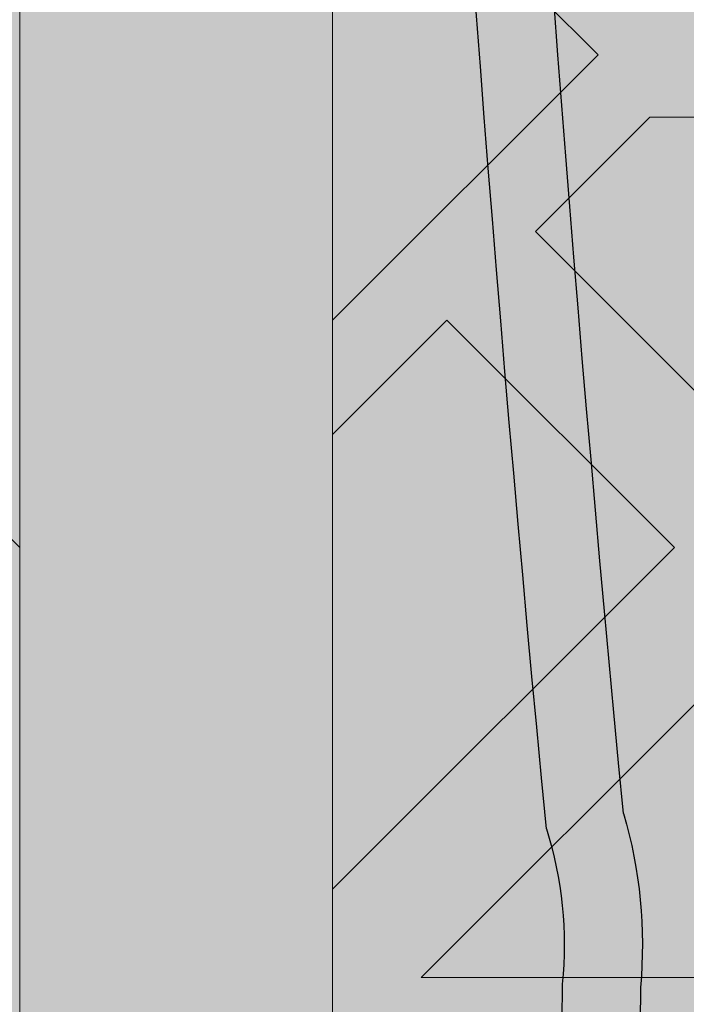
# Model space of a CAD drawing. Units: inches. Extents: x 844 to 2234, y 346 to 1084.
# Tile 70 of 93: x 1998.757 to 2000.116, y 694.327 to 696.335. Entities that reach past the tile are written whole.
import ezdxf

# ---------------------------------------------------------------- set-up
doc = ezdxf.new("R2010")
doc.units = ezdxf.units.IN
doc.header["$MEASUREMENT"] = 0
for name, color, linetype, lineweight in [('A-ANNO-DIMS', 2, 'Continuous', 18), ('furniture', 8, 'Continuous', 18), ('RA-AP-01$0$INT', 35, 'Continuous', 5)]:
    doc.layers.add(name, color=color, linetype=linetype, lineweight=lineweight)
doc.layers.add('RA-AP-01$0$FURN', color=3, linetype='Continuous')
doc.layers.add('RA-AP-01$0$WOOD', color=64, linetype='Continuous')
doc.styles.get("Standard").update_dxf_attribs({"font": 'arial.ttf'})
doc.dimstyles.get("Standard").update_dxf_attribs({"dimtxt": 6, "dimasz": 3, "dimexe": 0.18, "dimexo": 0.0625, "dimgap": 0.09, "dimtad": 0, "dimtih": 1, "dimtoh": 1, "dimdec": 1, "dimzin": 0, "dimdsep": 46, "dimlunit": 3, "dimtxsty": 'Standard', "dimblk": 'ARCHTICK', "dimcen": 0.09, "dimadec": 0, "dimazin": 0, "dimtfac": 1, "dimtdec": 1, "dimtofl": 0, "dimtmove": 0, "dimatfit": 3, "dimfxl": 1, "dimtolj": 1, "dimtzin": 0, "dimarcsym": 0})

# ---------------------------------------------------------------- blocks, each defined once
blk = doc.blocks.new('A$C18D01794')
at = {"layer": 'RA-AP-01$0$INT'}
h = blk.add_hatch(color=256, dxfattribs=at)
h.paths.add_polyline_path([(4.469348592586677, -7.07085414521094), (4.505206456958073, -7.03499628085108), (4.505206456958071, -7.106712009593861)])
h.paths.add_polyline_path([(4.455206456960671, -7.084996280832395), (4.476922185709333, -7.106712009588038), (4.433490728198045, -7.106712009588038)])
h.paths.add_polyline_path([(4.405206456958073, -7.034996280813718), (4.441064321339218, -7.070854145206393), (4.40520645695807, -7.106712009576003)])
h.paths.add_polyline_path([(4.425206456989053, -6.911460746921742), (4.455206456990736, -6.881460746929706), (4.485206456989055, -6.911460746937677), (4.48520645696979, -7.026712009590022), (4.455206456965227, -7.056712009584936), (4.425206456969784, -7.026712009579853)])
h.paths.add_polyline_path([(4.505206456958073, -6.831460746955388), (4.505206456958071, -6.903176475661116), (4.469348592616738, -6.867318611308251)])
h.paths.add_polyline_path([(4.425206456964688, -6.707925213036777), (4.455206456964794, -6.677925213027025), (4.485206456964689, -6.707925213017265), (4.485206456983951, -6.823176475683938), (4.455206456990736, -6.853176475686799), (4.425206456983956, -6.823176475689667)])
h.paths.add_polyline_path([(4.425206456974126, -6.504389679118949), (4.455206456959092, -6.474389679124341), (4.485206456974132, -6.504389679129721), (4.485206456993396, -6.619640941768059), (4.45520645699153, -6.649640941779566), (4.425206456993394, -6.619640941791077)])
h.paths.add_polyline_path([(4.46934859260189, -6.663783077416661), (4.505206456958071, -6.627925213048953), (4.505206456958073, -6.699640941761311)])
h.paths.add_polyline_path([(4.405206456958073, -6.627925213005104), (4.441064321354427, -6.663783077389926), (4.405206456958072, -6.699640941797813)])
h.paths.add_polyline_path([(4.405206456958072, -6.424389679139403), (4.441064321333084, -6.460247543502882), (4.405206456958072, -6.496105407889427)])
h.paths.add_polyline_path([(4.469348592580547, -6.460247543498336), (4.505206456958071, -6.424389679109282), (4.505206456958071, -6.496105407864332)])
h.paths.add_polyline_path([(4.425206456957888, -6.300854145208262), (4.45520645695415, -6.270854145221655), (4.485206456959507, -6.300854145217359), (4.48520645695824, -6.416105407863534), (4.455206456954537, -6.44610540787688), (4.425206456957888, -6.416105407889874)])
h.paths.add_polyline_path([(4.425206456957888, -6.226712009591025), (4.471064321332215, -6.226712009591025), (4.425206456957888, -6.272569873980103)])
h.paths.add_polyline_path([(4.499348592575121, -6.226712009591029), (4.636064321343707, -6.226712009591025), (4.666064321342317, -6.256712009589254), (4.636064321340932, -6.286712009591028), (4.499348592588945, -6.286712009591028), (4.469348592591685, -6.256712009584116)])
h.paths.add_polyline_path([(4.680206456964641, -6.270854145214393), (4.716064321337824, -6.306712009588038), (4.644348592591454, -6.306712009588038)])
h.paths.add_polyline_path([(4.644348592588108, -6.206712009588038), (4.716064321341167, -6.206712009588038), (4.680206456964637, -6.242569873964111)])
h.paths.add_polyline_path([(4.724348592586768, -6.226712009589824), (4.861064321340514, -6.226712009589824), (4.891064321340324, -6.256712009589255), (4.861064321340141, -6.286712009589827), (4.724348592587134, -6.286712009589821), (4.694348592586957, -6.256712009589254)])
h.paths.add_polyline_path([(4.905206456964143, -6.270854145212892), (4.941064321338827, -6.306712009588038), (4.869348592589457, -6.306712009588039)])
h.paths.add_polyline_path([(4.869348592586113, -6.206712009588038), (4.941064321342172, -6.206712009588038), (4.905206456964145, -6.242569873965612)])
h.paths.add_polyline_path([(4.949348592587774, -6.226712009589824), (5.086064321341521, -6.226712009589824), (5.116064321341329, -6.256712009589252), (5.08606432134115, -6.286712009589823), (4.949348592588145, -6.286712009589827), (4.919348592587961, -6.256712009589255)])
h.paths.add_polyline_path([(5.130206456963645, -6.270854145214393), (5.166064321336834, -6.306712009588038), (5.094348592590464, -6.306712009588038)])
h.paths.add_polyline_path([(5.094348592587119, -6.206712009588038), (5.166064321340178, -6.206712009588038), (5.130206456963651, -6.242569873964107)])
h.paths.add_polyline_path([(5.174348592584578, -6.226712009591027), (5.311064321353163, -6.226712009591027), (5.341064321336602, -6.256712009584116), (5.31106432133934, -6.286712009591028), (5.174348592587352, -6.286712009591028), (5.144348592585969, -6.256712009589254)])
h.paths.add_polyline_path([(5.325206456968778, -6.300854145217359), (5.355206456974136, -6.270854145221653), (5.385206456970396, -6.300854145208262), (5.385206456970396, -6.416105407889878), (5.355206456973747, -6.44610540787688), (5.325206456970044, -6.416105407863533)])
h.paths.add_polyline_path([(5.339348592596073, -6.226712009591029), (5.385206456970396, -6.226712009591025), (5.385206456970398, -6.272569873980105)])
h.paths.add_polyline_path([(5.325206456954155, -6.504389679129722), (5.355206456969194, -6.474389679124342), (5.38520645695416, -6.504389679118949), (5.385206456934896, -6.619640941791077), (5.355206456936758, -6.649640941779564), (5.325206456934888, -6.619640941768057)])
h.paths.add_polyline_path([(5.305206456958072, -6.424389679097139), (5.341064321347739, -6.460247543498338), (5.305206456958072, -6.496105407876472)])
h.paths.add_polyline_path([(5.369348592595204, -6.460247543502882), (5.40520645695807, -6.42438967915155), (5.405206456958072, -6.496105407877278)])
h.paths.add_polyline_path([(5.405206456958072, -6.627925213017245), (5.405206456958072, -6.69964094178567), (5.369348592573857, -6.663783077389926)])
h.paths.add_polyline_path([(5.305206456958072, -6.62792521303681), (5.341064321326393, -6.663783077416663), (5.305206456958072, -6.69964094177345)])
h.paths.add_polyline_path([(5.325206456963599, -6.707925213017267), (5.355206456963494, -6.677925213027021), (5.385206456963598, -6.707925213036775), (5.385206456944334, -6.823176475689665), (5.355206456937552, -6.853176475686797), (5.325206456944333, -6.823176475683936)])
h.paths.add_polyline_path([(5.305206456958072, -6.831460746943246), (5.341064321311551, -6.867318611308252), (5.305206456958072, -6.903176475673257)])
h.paths.add_polyline_path([(5.325206456939231, -6.911460746937672), (5.355206456937552, -6.881460746929707), (5.385206456939235, -6.911460746921742), (5.385206456958502, -7.026712009579853), (5.355206456963061, -7.056712009584934), (5.3252064569585, -7.026712009590026)])
h.paths.add_polyline_path([(5.404581768715993, -6.832085435167151, 0.001217816984214), (5.405206456958072, -6.832312009593747), (5.405206456958072, -6.90317647569123), (5.369348592563558, -6.867318611308251)])
h.paths.add_polyline_path([(5.36934859258907, -7.070854145206393), (5.40520645695807, -7.034996280825861), (5.405206456958072, -7.106712009563858)])
h.paths.add_polyline_path([(5.355206456967613, -7.084996280832394), (5.376922185730239, -7.106712009588038), (5.333490728218953, -7.106712009588036)])
h.paths.add_polyline_path([(5.30520645695807, -7.034996280838937), (5.341064321341609, -7.070854145210942), (5.305206456958074, -7.106712009606006)])
h = blk.add_hatch(color=256, dxfattribs=at)
h.paths.add_polyline_path([(4.505206456958071, -6.627925213048953), (4.46934859260189, -6.663783077416663), (4.505206456958071, -6.699640941761309), (4.505206456958071, -6.831460746955389), (4.469348592616735, -6.867318611308252), (4.505206456958071, -6.903176475661112), (4.505206456958071, -7.03499628085108), (4.469348592586679, -7.070854145210939), (4.505206456952245, -7.106712009588038), (4.476922185709333, -7.106712009588038), (4.455206456960671, -7.084996280832395), (4.433490728198047, -7.106712009588038), (4.405206456946033, -7.10671200958804), (4.441064321339216, -7.070854145206393), (4.40520645695807, -7.034996280813718), (4.405206456958072, -6.903176475703379), (4.441064321364728, -6.867318611308251), (4.40520645695807, -6.83146074691313), (4.40520645695807, -6.699640941797813), (4.441064321354429, -6.663783077389924), (4.405206456958072, -6.627925213005102), (4.405206456958072, -6.496105407889425), (4.441064321333084, -6.460247543502882), (4.405206456958072, -6.424389679139403), (4.405206456958072, -6.206712009588038), (4.644348592588106, -6.206712009588038), (4.680206456964639, -6.242569873964107), (4.716064321341165, -6.206712009588038), (4.869348592586113, -6.206712009588038), (4.905206456964143, -6.24256987396561), (4.941064321342174, -6.206712009588038), (5.094348592587118, -6.206712009588038), (5.130206456963649, -6.242569873964107), (5.166064321340178, -6.206712009588038), (5.405206456958072, -6.206712009588038), (5.405206456958072, -6.42438967915155), (5.369348592595202, -6.46024754350288), (5.40520645695807, -6.49610540787728), (5.40520645695807, -6.627925213017247), (5.369348592573859, -6.663783077389926), (5.40520645695807, -6.699640941785666), (5.40520645695807, -6.831460746925273), (5.36934859256356, -6.867318611308252), (5.405206456958072, -6.90317647569123), (5.405206456958072, -7.034996280825859), (5.369348592589068, -7.070854145206395), (5.405206456982249, -7.106712009588038), (5.376922185730244, -7.106712009588038), (5.355206456967613, -7.084996280832397), (5.333490728218955, -7.106712009588036), (5.305206456976043, -7.106712009588035), (5.341064321341609, -7.07085414521094), (5.305206456958072, -7.034996280838935), (5.305206456958072, -6.90317647567326), (5.34106432131155, -6.867318611308252), (5.305206456958072, -6.831460746943244), (5.30520645695807, -6.699640941773452), (5.341064321326395, -6.663783077416663), (5.305206456958072, -6.627925213036814), (5.305206456958072, -6.496105407876472), (5.341064321347738, -6.46024754349834), (5.305206456958072, -6.424389679097137), (5.30520645695807, -6.306712009588038), (5.166064321336834, -6.306712009588038), (5.130206456963647, -6.270854145214393), (5.094348592590464, -6.306712009588038), (4.941064321338827, -6.306712009588036), (4.905206456964145, -6.270854145212892), (4.869348592589459, -6.306712009588038), (4.716064321337822, -6.306712009588036), (4.680206456964641, -6.270854145214393), (4.644348592591453, -6.306712009588038), (4.505206456958071, -6.306712009588038), (4.505206456958071, -6.424389679109282), (4.469348592580545, -6.460247543498338), (4.505206456958071, -6.496105407864328)])
h.paths.add_polyline_path([(4.485206456974132, -6.504389679129722), (4.45520645695909, -6.474389679124341), (4.425206456974128, -6.504389679118945), (4.425206456993394, -6.619640941791079), (4.45520645699153, -6.649640941779566), (4.485206456993396, -6.619640941768059)], flags=16)
h.paths.add_polyline_path([(4.455206456954537, -6.44610540787688), (4.485206456958242, -6.416105407863534), (4.48520645695951, -6.30085414521736), (4.45520645695415, -6.270854145221653), (4.425206456957888, -6.300854145208264), (4.425206456957888, -6.41610540788988)], flags=16)
h.paths.add_polyline_path([(4.455206456964794, -6.677925213027025), (4.42520645696469, -6.707925213036777), (4.425206456983954, -6.82317647568967), (4.455206456990734, -6.853176475686797), (4.485206456983953, -6.823176475683936), (4.485206456964687, -6.707925213017265)], flags=16)
h.paths.add_polyline_path([(4.499348592588947, -6.286712009591028), (4.636064321340932, -6.286712009591028), (4.666064321342317, -6.256712009589254), (4.636064321343707, -6.226712009591027), (4.499348592575121, -6.226712009591029), (4.469348592591685, -6.256712009584118)], flags=16)
h.paths.add_polyline_path([(4.425206456957888, -6.272569873980103), (4.471064321332215, -6.226712009591025), (4.425206456957888, -6.226712009591025)], flags=16)
h.paths.add_polyline_path([(4.455206456990734, -6.881460746929709), (4.425206456989053, -6.91146074692174), (4.425206456969784, -7.026712009579853), (4.455206456965226, -7.056712009584932), (4.485206456969787, -7.026712009590026), (4.485206456989053, -6.911460746937672)], flags=16)
h.paths.add_polyline_path([(4.72434859258714, -6.286712009589821), (4.861064321340141, -6.286712009589829), (4.891064321340324, -6.256712009589254), (4.861064321340513, -6.226712009589823), (4.724348592586768, -6.226712009589823), (4.694348592586956, -6.256712009589254)], flags=16)
h.paths.add_polyline_path([(4.919348592587961, -6.256712009589254), (4.949348592588145, -6.286712009589827), (5.08606432134115, -6.286712009589823), (5.116064321341327, -6.256712009589254), (5.086064321341519, -6.226712009589824), (4.949348592587774, -6.226712009589824)], flags=16)
h.paths.add_polyline_path([(5.144348592585967, -6.256712009589254), (5.174348592587358, -6.286712009591028), (5.311064321339338, -6.286712009591028), (5.3410643213366, -6.256712009584118), (5.311064321353163, -6.226712009591029), (5.174348592584576, -6.226712009591027)], flags=16)
h.paths.add_polyline_path([(5.32520645693489, -6.619640941768055), (5.355206456936755, -6.649640941779566), (5.385206456934894, -6.619640941791079), (5.38520645695416, -6.504389679118949), (5.355206456969194, -6.474389679124341), (5.325206456954153, -6.504389679129724)], flags=16)
h.paths.add_polyline_path([(5.325206456970042, -6.416105407863534), (5.355206456973747, -6.44610540787688), (5.385206456970398, -6.416105407889876), (5.385206456970398, -6.30085414520826), (5.355206456974136, -6.270854145221653), (5.325206456968778, -6.30085414521736)], flags=16)
h.paths.add_polyline_path([(5.325206456963599, -6.707925213017265), (5.325206456944333, -6.823176475683936), (5.355206456937552, -6.853176475686797), (5.385206456944332, -6.823176475689667), (5.385206456963596, -6.707925213036773), (5.355206456963492, -6.677925213027027)], flags=16)
h.paths.add_polyline_path([(5.32520645693923, -6.911460746937674), (5.3252064569585, -7.026712009590026), (5.355206456963062, -7.056712009584934), (5.3852064569585, -7.026712009579853), (5.385206456939234, -6.911460746921738), (5.355206456937552, -6.881460746929707)], flags=16)
h.paths.add_polyline_path([(5.339348592596071, -6.226712009591029), (5.385206456970398, -6.272569873980103), (5.385206456970396, -6.226712009591027)], flags=16)
blk.add_hatch(color=256, dxfattribs=at).paths.add_polyline_path([(4.505206456958071, -6.306712009588038), (5.305206456958072, -6.306712009588038), (5.305206456958072, -7.106712009588038), (5.255206456951893, -7.10671200958804), (5.25520645694868, -6.356712009605972), (4.555206456959269, -6.356712009587461), (4.555206456956052, -7.106712009588038), (4.505206456958073, -7.106712009588038)])
h = blk.add_hatch(color=256, dxfattribs=at)
h.paths.add_polyline_path([(4.585917135068448, -6.356712009588273), (4.614201406330596, -6.356712009589021), (4.668846067270487, -6.411356670531338), (4.723490728212344, -6.356712009591912), (4.771774999457151, -6.35671200959319), (4.826419660396886, -6.411356670535356), (4.862780050090322, -6.374996280843536), (4.844495778842715, -6.356712009595112), (4.862780050090411, -6.356712009595595), (4.905206456960182, -6.399138416468211), (4.947632863832445, -6.356712009597838), (4.965917135079675, -6.356712009598322), (4.947632863831759, -6.374996280845421), (4.983993253523576, -6.411356670538857), (5.038637914464627, -6.356712009600247), (5.08692218571208, -6.356712009601523), (5.141566846649976, -6.411356670541852), (5.196211507589851, -6.356712009604411), (5.224495778822615, -6.356712009605161), (4.905206456953975, -6.676001331473793)])
h.paths.add_polyline_path([(4.895206456956031, -6.637717060225675), (4.895206456958921, -6.528427738347902), (4.840561796018589, -6.583072399285802)], flags=16)
h.paths.add_polyline_path([(4.915206456955638, -6.637717060226121), (4.969851117895509, -6.583072399288678), (4.915206456957609, -6.528427738348344)], flags=16)
h.paths.add_polyline_path([(4.826419660395175, -6.568930263661755), (4.881064321335613, -6.514285602723745), (4.771774999456703, -6.514285602720857)], flags=16)
h.paths.add_polyline_path([(4.983993253519558, -6.568930263665262), (5.038637914460456, -6.514285602726792), (4.929348592581548, -6.514285602724816)], flags=16)
h.paths.add_polyline_path([(4.881064321336025, -6.494285602723742), (4.826419660397532, -6.439640941782821), (4.771774999457062, -6.494285602720859)], flags=16)
h.paths.add_polyline_path([(4.929348592582019, -6.494285602724817), (5.038637914460982, -6.494285602726792), (4.983993253522945, -6.439640941786327)], flags=16)
h.paths.add_polyline_path([(4.895206456960191, -6.480143467100443), (4.895206456962115, -6.407422687715913), (4.876922185715016, -6.389138416467584), (4.840561796021581, -6.425498806159401)], flags=16)
h.paths.add_polyline_path([(4.915206456958487, -6.480143467100889), (4.969851117899527, -6.425498806162279), (4.933490728206909, -6.389138416468043), (4.9152064569598, -6.40742268771434)], flags=16)
h.paths.add_polyline_path([(4.757632863832376, -6.480143467096812), (4.812277524772842, -6.425498806158772), (4.757632863834348, -6.370854145217844)], flags=16)
h.paths.add_polyline_path([(4.737632863832376, -6.480143467096286), (4.737632863834348, -6.370854145217375), (4.682988202893906, -6.425498806155385)], flags=16)
h.paths.add_polyline_path([(5.05278005008503, -6.480143467103376), (5.052780050087917, -6.370854145224413), (4.998135389146995, -6.425498806162908)], flags=16)
h.paths.add_polyline_path([(5.072780050085024, -6.480143467103744), (5.127424711025931, -6.42549880616527), (5.072780050087916, -6.370854145224832)], flags=16)
h.paths.add_polyline_path([(4.935917135072783, -6.706712009592292), (5.255206456948811, -6.387422687716309), (5.255206456948932, -6.415706958964177), (5.200561796010279, -6.470351619902839), (5.255206456949403, -6.524996280841948), (5.25520645694961, -6.5732805520894), (5.200561796009787, -6.627925213029239), (5.236922185702417, -6.664285602721864), (5.255206456949919, -6.646001331474357), (5.255206456949998, -6.664285602721898), (5.212780050078687, -6.706712009592262), (5.25520645695036, -6.749138416463932), (5.255206456950438, -6.767422687711313), (5.236922185702424, -6.749138416463297), (5.200561796009796, -6.785498806155928), (5.255206456950753, -6.840143467096874), (5.25520645695096, -6.888427738341682), (5.200561796010322, -6.943072399282328), (5.255206456951428, -6.997717060223427), (5.255206456951547, -7.026001331471006)])
h.paths.add_polyline_path([(5.042988202883395, -6.785498806155427), (5.097632863823085, -6.840143467095101), (5.097632863822622, -6.730854145216193)], flags=16)
h.paths.add_polyline_path([(5.028846067259663, -6.771356670531693), (5.083490728198774, -6.716712009592573), (4.974201406321001, -6.716712009593042)], flags=16)
h.paths.add_polyline_path([(5.117632863823087, -6.840143467095186), (5.172277524762331, -6.785498806155926), (5.11763286382262, -6.730854145216225)], flags=16)
h.paths.add_polyline_path([(5.08349072819877, -6.696712009593886), (5.028846067259652, -6.642067348654775), (4.974201406320998, -6.696712009593438)], flags=16)
h.paths.add_polyline_path([(5.131774999446817, -6.854285602718917), (5.186419660386065, -6.799640941779662), (5.241064321325782, -6.854285602719365)], flags=17)
h.paths.add_polyline_path([(5.131774999446228, -6.716712009592374), (5.186419660386065, -6.771356670532194), (5.222780050079488, -6.734996280838764), (5.204495778832781, -6.716712009592063)], flags=16)
h.paths.add_polyline_path([(5.097632863822613, -6.682569873970264), (5.097632863823061, -6.573280552091354), (5.042988202883383, -6.627925213031044)], flags=16)
h.paths.add_polyline_path([(5.131774999446899, -6.874285602718915), (5.241064321325809, -6.874285602719364), (5.186419660386591, -6.928930263658598)], flags=17)
h.paths.add_polyline_path([(5.131774999446226, -6.696712009594078), (5.204495778830767, -6.696712009594374), (5.22278005007868, -6.67842773834687), (5.186419660386049, -6.642067348654249)], flags=16)
h.paths.add_polyline_path([(5.11763286382262, -6.682569873970225), (5.17227752476232, -6.627925213030515), (5.117632863823064, -6.573280552091267)], flags=16)
h.paths.add_polyline_path([(5.186419660386069, -6.613783077405491), (5.241064321325754, -6.559138416465795), (5.131774999446791, -6.559138416466263)], flags=16)
h.paths.add_polyline_path([(5.131774999446872, -6.539138416466263), (5.24106432132578, -6.539138416465794), (5.186419660386554, -6.484493755526573)], flags=16)
h.paths.add_polyline_path([(5.255206456951811, -7.08742268770861), (5.255206456951895, -7.106712009588038), (4.555206456956052, -7.106712009588038), (4.555206456956136, -7.087422687708617), (4.905206456953973, -6.737422687710788)])
h.paths.add_polyline_path([(4.983993253513404, -6.8444937555241), (4.92934859257295, -6.899138416462108), (5.03863791445186, -6.899138416465014)], flags=16)
h.paths.add_polyline_path([(4.969851117889988, -6.83035161990006), (4.915206456952556, -6.775706958960171), (4.915206456949648, -6.884996280837944)], flags=16)
h.paths.add_polyline_path([(4.929348592572535, -6.919138416462105), (4.983993253511019, -6.973783077403037), (5.038637914451496, -6.919138416465012)], flags=16)
h.paths.add_polyline_path([(5.052780050074912, -6.93328055208906), (4.998135389134438, -6.987925213027088), (5.052780050072919, -7.042569873968025)], flags=16)
h.paths.add_polyline_path([(5.07278005007491, -6.933280552089588), (5.072780050072918, -7.042569873968497), (5.127424711013374, -6.987925213030498)], flags=16)
h.paths.add_polyline_path([(4.89520645695295, -6.775706958959721), (4.840561796013067, -6.830351619897157), (4.895206456950961, -6.884996280837494)], flags=16)
h.paths.add_polyline_path([(4.915206456948365, -6.933280552085403), (4.915206456946434, -7.006001331471951), (4.933490728192729, -7.024285602719066), (4.969851117886972, -6.987925213026453)], flags=16)
h.paths.add_polyline_path([(4.881064321327021, -6.899138416461022), (4.82641966038902, -6.84449375552057), (4.771774999448108, -6.899138416459029)], flags=16)
h.paths.add_polyline_path([(4.895206456950073, -6.933280552084951), (4.840561796009022, -6.987925213023558), (4.876922185700835, -7.024285602716997), (4.895206456948749, -7.006001331469487)], flags=16)
h.paths.add_polyline_path([(4.983993253510392, -7.0020673486505), (4.947632863816944, -7.038427738342319), (4.965917135064043, -7.05671200959023), (5.038637914448995, -7.056712009591555)], flags=16)
h.paths.add_polyline_path([(4.881064321326543, -6.91913841646102), (4.771774999447578, -6.919138416459031), (4.826419660385607, -6.973783077399508)], flags=16)
h.paths.add_polyline_path([(4.905206456946447, -7.014285602717636), (4.862780050074785, -7.056712009588352), (4.947632863816685, -7.056712009589775)], flags=16)
h.paths.add_polyline_path([(5.14156684663679, -7.002067348654549), (5.086922185696452, -7.056712009592438), (5.196211507574223, -7.056712009594425)], flags=16)
h.paths.add_polyline_path([(4.8264196603837, -7.002067348646972), (4.771774999442643, -7.056712009585575), (4.8444957788276, -7.056712009587508), (4.862780050075511, -7.038427738340416)], flags=16)
h.paths.add_polyline_path([(4.812277524760289, -6.98792521302292), (4.757632863822258, -6.933280552082447), (4.757632863819352, -7.042569873961408)], flags=16)
h.paths.add_polyline_path([(4.73763286382226, -6.933280552082079), (4.682988202881349, -6.987925213020536), (4.737632863819352, -7.04256987396099)], flags=16)
h.paths.add_polyline_path([(4.723490728195188, -7.056712009584289), (4.668846067257299, -7.002067348643949), (4.614201406317417, -7.056712009581383)], flags=16)
h.paths.add_polyline_path([(4.597632863829262, -6.706712009592262), (4.555206456957951, -6.664285602721896), (4.555206456958029, -6.646001331474357), (4.573490728205535, -6.664285602721864), (4.609851117898167, -6.627925213029238), (4.555206456958338, -6.573280552089402), (4.555206456958546, -6.524996280841952), (4.60985111789767, -6.470351619902839), (4.555206456959015, -6.415706958964177), (4.555206456959138, -6.387422687716309), (4.874495778835167, -6.70671200959229), (4.5552064569564, -7.026001331471015), (4.555206456956523, -6.997717060223433), (4.609851117897629, -6.94307239928233), (4.555206456956988, -6.888427738341681), (4.555206456957198, -6.840143467096881), (4.609851117898153, -6.78549880615593), (4.573490728205528, -6.749138416463297), (4.555206456957507, -6.76742268771132), (4.555206456957585, -6.749138416463933)])
h.paths.add_polyline_path([(4.712780050085332, -6.730854145216195), (4.712780050084863, -6.840143467095105), (4.767424711024555, -6.785498806155427)], flags=16)
h.paths.add_polyline_path([(4.726922185709173, -6.716712009592573), (4.781566846648288, -6.771356670531693), (4.836211507586949, -6.716712009593043)], flags=16)
h.paths.add_polyline_path([(4.692780050085327, -6.730854145216225), (4.638135389145619, -6.785498806155928), (4.692780050084865, -6.840143467095185)], flags=16)
h.paths.add_polyline_path([(4.726922185709182, -6.696712009593886), (4.836211507586949, -6.696712009593436), (4.7815668466483, -6.642067348654773)], flags=16)
h.paths.add_polyline_path([(4.678637914461726, -6.71671200959237), (4.605917135075169, -6.716712009592063), (4.587632863828464, -6.734996280838766), (4.623993253521887, -6.771356670532195)], flags=16)
h.paths.add_polyline_path([(4.712780050085336, -6.68256987397026), (4.767424711024568, -6.627925213031042), (4.71278005008489, -6.573280552091352)], flags=16)
h.paths.add_polyline_path([(4.678637914461726, -6.696712009594076), (4.623993253521899, -6.642067348654247), (4.587632863829271, -6.67842773834687), (4.605917135077185, -6.696712009594376)], flags=16)
h.paths.add_polyline_path([(4.692780050085336, -6.682569873970228), (4.692780050084889, -6.573280552091267), (4.638135389145632, -6.627925213030515)], flags=16)
h.paths.add_polyline_path([(4.623993253521885, -6.799640941779662), (4.678637914461131, -6.854285602718915), (4.56934859258217, -6.854285602719365)], flags=17)
h.paths.add_polyline_path([(4.623993253521901, -6.613783077405509), (4.678637914461158, -6.559138416466263), (4.569348592582195, -6.559138416465795)], flags=16)
h.paths.add_polyline_path([(4.678637914461051, -6.874285602718915), (4.623993253521361, -6.928930263658598), (4.569348592582143, -6.874285602719364)], flags=17)
h.paths.add_polyline_path([(4.678637914461076, -6.539138416466263), (4.623993253521399, -6.484493755526573), (4.569348592582167, -6.539138416465796)], flags=16)
h = blk.add_hatch(color=256, dxfattribs=at)
h.paths.add_polyline_path([(5.028846067259997, -6.642067348655121), (4.974201406321342, -6.696712009593783), (5.083490728199115, -6.69671200959423)])
h.paths.add_polyline_path([(4.974201406321344, -6.716712009593388), (5.028846067260004, -6.771356670532039), (5.083490728199117, -6.716712009592919)])
h.paths.add_polyline_path([(5.042988202883738, -6.785498806155768), (5.097632863823428, -6.840143467095449), (5.097632863822963, -6.73085414521654)])
h.paths.add_polyline_path([(5.117632863822961, -6.730854145216568), (5.117632863823428, -6.840143467095531), (5.172277524762674, -6.785498806156272)])
h.paths.add_polyline_path([(5.131774999446572, -6.716712009592718), (5.186419660386406, -6.77135667053254), (5.222780050079831, -6.734996280839116), (5.204495778833122, -6.716712009592409)])
h.paths.add_polyline_path([(5.236922185702764, -6.749138416463644), (5.200561796010139, -6.785498806156274), (5.255206456949971, -6.840143467096101), (5.255206456950271, -6.76742268771115)])
h.paths.add_polyline_path([(5.186419660386412, -6.799640941780006), (5.131774999447164, -6.854285602719262), (5.241064321326123, -6.854285602719711)])
h.paths.add_polyline_path([(5.131774999447238, -6.874285602719261), (5.186419660386934, -6.928930263658944), (5.241064321326153, -6.874285602719709)])
h.paths.add_polyline_path([(5.200561796010663, -6.943072399282675), (5.255206456949324, -6.997717060221329), (5.255206456949777, -6.888427738343558)])
h.paths.add_polyline_path([(5.21278005007903, -6.706712009592607), (5.255206456950223, -6.749138416463798), (5.255206456950696, -6.664285602721891)])
h.paths.add_polyline_path([(5.13177499944657, -6.696712009594424), (5.204495778831106, -6.696712009594723), (5.222780050079024, -6.678427738347219), (5.186419660386397, -6.642067348654592)])
h.paths.add_polyline_path([(5.117632863823405, -6.573280552091611), (5.117632863822955, -6.682569873970578), (5.172277524762665, -6.627925213030859)])
h.paths.add_polyline_path([(5.042988202883727, -6.627925213031387), (5.097632863822957, -6.682569873970603), (5.097632863823407, -6.573280552091697)])
h.paths.add_polyline_path([(5.131774999447135, -6.559138416466609), (5.186419660386394, -6.613783077405857), (5.241064321326097, -6.559138416466144)])
h.paths.add_polyline_path([(5.200561796010128, -6.627925213029584), (5.236922185702758, -6.664285602722211), (5.255206456950264, -6.646001331474705), (5.255206456949948, -6.573280552089752)])
h.paths.add_polyline_path([(5.186419660386895, -6.484493755526919), (5.131774999447213, -6.539138416466609), (5.241064321326127, -6.539138416466142)])
h.paths.add_polyline_path([(5.200561796010624, -6.470351619903183), (5.255206456949745, -6.524996280842298), (5.255206456949276, -6.415706958964523)])
for p, q in [((5.255206456951895, -7.106712009588038), (5.255206456948681, -6.356712009605972)), ((5.131774999446792, -6.559138416466263), (5.241064321325755, -6.559138416465795)), ((5.241064321325755, -6.559138416465795), (5.186419660386049, -6.613783077405509)), ((5.255206456949605, -6.573280552089405), (5.200561796009783, -6.627925213029239)), ((5.255206456949918, -6.646001331474357), (5.255206456949605, -6.573280552089405)), ((5.200561796009783, -6.627925213029238), (5.236922185702415, -6.664285602721863)), ((5.305206456939818, -6.627925213018556), (5.341064321310754, -6.663783077401021)), ((5.186419660386051, -6.642067348654247), (5.222780050078681, -6.67842773834687)), ((5.255206456949919, -6.646001331474357), (5.236922185702415, -6.664285602721864)), ((5.212780050078687, -6.706712009592262), (5.255206456950353, -6.664285602721543)), ((5.25520645694988, -6.74913841646345), (5.255206456950353, -6.664285602721543)), ((5.204495778833082, -6.69671200959206), (5.222780050078681, -6.67842773834687)), ((5.204495778831179, -6.696712009594376), (5.131774999446228, -6.696712009594078)), ((5.212780050078687, -6.706712009592262), (5.25520645694988, -6.74913841646345))]:
    blk.add_line(p, q, dxfattribs=at)
blk.add_lwpolyline([(5.305206456958072, -7.106712009588038), (5.305206456958072, -6.306712009588038), (4.505206456958071, -6.306712009588038), (4.505206456958071, -7.106712009588038)], dxfattribs=at)
blk = doc.blocks.new('A$C32926AE1')
at = {"layer": 'RA-AP-01$0$WOOD'}
h = blk.add_hatch(color=256, dxfattribs=at)
h.dxf.hatch_style = 1
h.paths.add_polyline_path([(5.157430609644524, 4.573483066760929, -0.1009492694046607), (5.155401577623758, 4.593365984175333, -0.1842662638101597), (5.172249623284174, 4.638795604568598, 0.2056608120311276), (5.179560981299304, 4.661316324430096, 0.3614336704623542), (5.134352340494423, 4.706524965234944, 0.2056608120311297), (5.111831620632933, 4.699213607219793, -0.1842662638101113), (5.066402000239693, 4.682365561559342, -0.1055311479399994), (5.045656153913092, 4.68467289944697, 0.1567636581983829), (4.763886414745334, 4.684672899446966, -0.1055311479399895), (4.743140568418733, 4.68236556155934, -0.1842662638100833), (4.6977109480255, 4.69921360721979, 0.2056608120302612), (4.675190228164109, 4.706524965234949, 0.3614336704708441), (4.629981587358889, 4.66131632442871, 0.2056608120245944), (4.637292945374126, 4.638795604567974, -0.1842662638101024), (4.654140991034615, 4.59336598417475, -0.1009492694055169), (4.652111959013835, 4.573483066760181, 0.021410119221476), (4.629748025606143, 4.156712009541676, 0.0214101192214795), (4.652111959013809, 3.739940952323101, -0.1009492694059586), (4.654140991034615, 3.720058034908448, -0.1842662638100975), (4.637292945374126, 3.674628414515226, 0.2056608120245705), (4.629981587358889, 3.652107694654492, 0.3614336704708879), (4.675190228164113, 3.606899053848249, 0.2056608120302384), (4.697710948025501, 3.614210411863408, -0.1842662638100995), (4.743140568418738, 3.63105845752386, -0.1055311479402541), (4.763886414745388, 3.628751119636215, 0.1567636581983776), (5.045656153913137, 3.628751119636244, -0.1055311479397538), (5.066402000239692, 3.631058457523857, -0.1842662638101067), (5.111831620632931, 3.614210411863407, 0.2056608120310924), (5.134352340494417, 3.606899053848256, 0.3614336704624001), (5.179560981299307, 3.652107694653103, 0.2056608120311314), (5.172249623284175, 3.6746284145146, -0.1842662638101402), (5.155401577623758, 3.72005803490786, -0.1009492694051366), (5.15743060964455, 3.739940952322354, 0.0214101192215073), (5.179794543052287, 4.156712009541468, 0.0214101192215252)])
h.paths.add_polyline_path([(4.639748609479751, 4.156712009541513, 0.0213537860821624), (4.661970494867118, 3.741887061152232, -0.094075836301374), (4.664143710413708, 3.7196126951003, -0.1824818158568985), (4.644813765429836, 3.668037719127816, 0.2056608120245319), (4.639939526753007, 3.653023905887301, 0.3614336704710246), (4.676106439397173, 3.616856993242342, 0.2056608120302234), (4.691120252638095, 3.621731231919122, -0.1824818158602558), (4.742695228611606, 3.641061176902986, -0.1029891339458722), (4.766991894714349, 3.638256818950944, 0.156709409989566), (5.042550673941472, 3.638256818950105, -0.102989133958497), (5.066847340047078, 3.641061176902949, -0.1824818158594995), (5.118422316020358, 3.621731231919103, 0.2056608120311416), (5.133436129261316, 3.616856993242346, 0.3614336704621468), (5.169603041905217, 3.653023905886178, 0.2056608120310986), (5.164728803228477, 3.668037719127177, -0.1824818158565612), (5.145398858244737, 3.719612695099578, -0.0940758363009313), (5.147572073791232, 3.741887061151398, 0.0213537860822023), (5.169793959178681, 4.156712009541451, 0.0213537860822226), (5.147572073791203, 4.571536957931898, -0.0940758363005034), (5.145398858244737, 4.59381132398362, -0.1824818158565587), (5.164728803228476, 4.645386299956021, 0.2056608120311045), (5.169603041905216, 4.66040011319702, 0.3614336704621845), (5.133436129261313, 4.696567025840856, 0.2056608120310773), (5.118422316020359, 4.691692787164098, -0.182481815859508), (5.066847340047078, 4.67236284218025, -0.1029891339584606), (5.04255067394148, 4.675167200133092, 0.156709409989566), (4.766991894714357, 4.675167200132257, -0.1029891339458842), (4.742695228611611, 4.672362842180213, -0.1824818158602725), (4.691120252638095, 4.691692787164077, 0.2056608120302152), (4.676106439397174, 4.696567025840858, 0.3614336704710363), (4.639939526753005, 4.660400113195899, 0.2056608120245495), (4.644813765429837, 4.645386299955384, -0.1824818158568934), (4.664143710413708, 4.593811323982902, -0.0940758363009187), (4.661970494867149, 4.571536957931074, 0.021353786082177)], flags=16)
h.paths.add_polyline_path([(5.129794543052235, 4.432167055276933, -0.0141661062790638), (5.130152669293814, 4.156927903047693, -0.0141661062790647), (5.129794543052234, 3.881688750818433, -0.0785247771143638), (5.10979738006795, 3.755143611847103, 0.0945969212073497), (5.105408519571111, 3.717898134952927, 0.1043170707844957), (5.116074640131521, 3.670385395016088, 0.1043170707864965), (5.068561900193738, 3.681051515576561, 0.09459692119553), (5.031316423304057, 3.676662655080835, -0.1580239521427272), (4.778226145355827, 3.676662655080367, 0.0945969211986668), (4.740980668464973, 3.681051515576592, 0.1043170707882822), (4.693467928526415, 3.670385395015844, 0.1043170707867916), (4.704134049087309, 3.717898134953662, 0.0945969211972894), (4.69974518859162, 3.755143611844042, -0.0785247771163196), (4.679748025606343, 3.881688750818406, -0.0141661062790663), (4.679389899364763, 4.156927903047693, -0.0141661062790672), (4.679748025606343, 4.432167055276998, -0.0785247771163064), (4.699745188591625, 4.55871219425134, 0.094596921197333), (4.704134049087308, 4.595957671141738, 0.1043170707867205), (4.693467928526416, 4.643470411079523, 0.1043170707882628), (4.740980668464965, 4.632804290518776, 0.0945969211988114), (4.778226145355874, 4.637193151015016, -0.158023952142669), (5.031316423304015, 4.637193151014546, 0.0945969211956361), (5.068561900193736, 4.632804290518806, 0.1043170707864979), (5.11607464013152, 4.643470411079278, 0.1043170707844617), (5.105408519571112, 4.595957671142455, 0.0945969212074597), (5.109797380067959, 4.558712194248236, -0.0785247771143467)], flags=0)
h.paths.add_polyline_path([(5.119794532311105, 4.432259799204851, -0.0142000800617244), (5.120156169157484, 4.156927903047701, -0.0142000800617277), (5.119794532311105, 3.881596006890482, -0.0784894509520253), (5.100273383573699, 3.758192358677797, 0.0940138827242913), (5.095413455884425, 3.717477693979438, 0.0606271852308753), (5.099615656341024, 3.686844378806616, 0.0606271852322524), (5.068982341167493, 3.691046579263239, 0.0940138827010453), (5.028267676478798, 3.686186651576848, -0.1580706864508061), (4.781274892180912, 3.686186651576435, 0.0940138827026903), (4.740560227491556, 3.691046579263279, 0.0606271852339895), (4.709926912317155, 3.686844378806508, 0.0606271852329405), (4.714129112773991, 3.717477693980356, 0.094013882701304), (4.709269185087677, 3.758192358669163, -0.0784894509577193), (4.689748036347473, 3.881596006890469, -0.014200080061729), (4.689386399501094, 4.156927903047709, -0.0142000800617217), (4.689748036347473, 4.432259799204808, -0.078489450957724), (4.709269185087651, 4.555663447426125, 0.0940138827014585), (4.714129112773992, 4.596378112114996, 0.0606271852329731), (4.709926912317154, 4.62701142728886, 0.0606271852340196), (4.74056022749157, 4.622809226832087, 0.0940138827024997), (4.781274892180847, 4.627669154518912, -0.1580706864508359), (5.028267676478777, 4.627669154518526, 0.0940138827010946), (5.068982341167492, 4.622809226832129, 0.060627185232254), (5.099615656341024, 4.627011427288751, 0.0606271852308727), (5.095413455884425, 4.59637811211593, 0.0940138827241088), (5.100273383573675, 4.555663447417647, -0.0784894509520978)], flags=0)
h.paths.add_polyline_path([(5.06978912287499, 4.430218106756144, -0.014241683694547), (5.070173729147532, 4.156927903047672, -0.0142416836945458), (5.06978912287499, 3.883637699339223, -0.0800609523125196), (5.052662118612511, 3.773463122773442, 0.0526421978001116), (5.04590916754064, 3.740550867606997, 0.0526421977992423), (5.012996912374707, 3.73379791653534, -0.1583028414718258), (4.796545656286308, 3.73379791653451, 0.0526421978034211), (4.763633401117837, 3.740550867607021, 0.0526421978018622), (4.756880450045755, 3.773463122774558, -0.0800609523117106), (4.739753445783639, 3.883637699339268, -0.0142416836945435), (4.739368839511098, 4.156927903047671, -0.0142416836945477), (4.739753445783639, 4.430218106756155, -0.0800609523116345), (4.75688045004574, 4.540392683320762, 0.052642197801941), (4.763633401117837, 4.573304938488346, 0.0526421978035071), (4.796545656286361, 4.580057889560873, -0.1583028414717561), (5.012996912374669, 4.580057889560039, 0.0526421977993048), (5.04590916754064, 4.57330493848837, 0.0526421978002057), (5.052662118612529, 4.540392683321868, -0.080060952312477)], flags=0)
h.paths.add_polyline_path([(5.049789715110557, 4.43038092723357, -0.0143097550741839), (5.05018085590259, 4.156927903047715, -0.0143097550741854), (5.049789715110558, 3.883474878861827, -0.0800685599149176), (5.03362098255317, 3.779581877367999, 0.0306258898956367), (5.028241146483733, 3.758218888663947, 0.0306258898977031), (5.006878157778253, 3.75283905259408, -0.1583983521624096), (4.802664410878162, 3.752839052594731, 0.0306258898946014), (4.781301422174808, 3.758218888663924, 0.0306258898967912), (4.775921586105202, 3.779581877368794, -0.080068559914251), (4.759752853548071, 3.883474878861786, -0.0143097550741854), (4.759361712756037, 4.156927903047671, -0.0143097550741854), (4.759752853548071, 4.430380927233557, -0.0800685599142479), (4.775921586105193, 4.534273928726546, 0.0306258898968306), (4.781301422174808, 4.555636917431444, 0.0306258898945754), (4.802664410878143, 4.561016753500631, -0.1583983521624168), (5.006878157778244, 4.561016753501291, 0.0306258898977177), (5.028241146483733, 4.555636917431421, 0.0306258898958182), (5.03362098255321, 4.534273928727244, -0.080068559914796)], flags=0)
h.paths.add_polyline_path([(4.999766070382627, 4.428171244713864, -0.0143443147609634), (5.000198441819402, 4.156927903047689, -0.0143443147609612), (4.999766070382627, 3.885684561381556, -0.0784641635803329), (4.987356730658798, 3.799103304488872, -0.1506053783831347), (4.822185837999821, 3.79910330448882, -0.0784641635803318), (4.809776498276007, 3.885684561381509, -0.014344314760963), (4.809344126839227, 4.156927903047677, -0.0143443147609645), (4.809776498276007, 4.428171244713873, -0.0784641635803192), (4.822185837999822, 4.514752501606549, -0.1506053783831338), (4.987356730658798, 4.514752501606494, -0.078464163580285)], flags=0)
h.paths.add_polyline_path([(4.979755254238824, 4.42764379880488, -0.0143772539198268), (4.980205517789977, 4.156927903047693, -0.0143772539198275), (4.979755254238824, 3.886212007290489, -0.0689242507424422), (4.971183264704897, 3.815276770442801, -0.1296645318904179), (4.838359303953726, 3.815276770442746, -0.0689242507424186), (4.829787314419809, 3.886212007290419, -0.0143772539198292), (4.829337050868653, 4.156927903047653, -0.0143772539198325), (4.829787314419809, 4.427643798804946, -0.0689242507424211), (4.838359303953725, 4.498579035652621, -0.1296645318904187), (4.971183264704897, 4.498579035652565, -0.0689242507424401)], flags=0)
h = blk.add_hatch(color=256, dxfattribs=at)
h.dxf.hatch_style = 1
h.paths.add_polyline_path([(5.145398858244737, 4.59381132398362, -0.1824818158565616), (5.164728803228476, 4.645386299956021, 0.2056608120311045), (5.169603041905216, 4.66040011319702, 0.3614336704621845), (5.133436129261313, 4.696567025840856, 0.2056608120310773), (5.118422316020359, 4.691692787164098, -0.182481815859508), (5.066847340047078, 4.67236284218025, -0.1029891339584606), (5.04255067394148, 4.675167200133092, 0.156709409989566), (4.766991894714357, 4.675167200132257, -0.1029891339458842), (4.742695228611611, 4.672362842180213, -0.1824818158602725), (4.691120252638095, 4.691692787164077, 0.2056608120302152), (4.676106439397174, 4.696567025840858, 0.3614336704710363), (4.639939526753005, 4.660400113195899, 0.2056608120245495), (4.644813765429837, 4.645386299955384, -0.1824818158568934), (4.664143710413708, 4.593811323982902, -0.0940758363009187), (4.661970494867149, 4.571536957931074, 0.0213537860821772), (4.639748609479751, 4.156712009541507, 0.0213537860821625), (4.661970494867119, 3.741887061152226, -0.0940758363013071), (4.664143710413708, 3.719612695100309, -0.1824818158569294), (4.644813765429836, 3.668037719127816, 0.2056608120245319), (4.639939526753007, 3.653023905887301, 0.3614336704710246), (4.676106439397173, 3.616856993242342, 0.2056608120302234), (4.691120252638095, 3.621731231919122, -0.1824818158602558), (4.742695228611606, 3.641061176902986, -0.1029891339458722), (4.766991894714349, 3.638256818950944, 0.156709409989566), (5.042550673941472, 3.638256818950105, -0.102989133958497), (5.066847340047078, 3.641061176902949, -0.1824818158594995), (5.118422316020358, 3.621731231919103, 0.2056608120311416), (5.133436129261316, 3.616856993242346, 0.3614336704621468), (5.169603041905217, 3.653023905886178, 0.2056608120310986), (5.164728803228477, 3.668037719127177, -0.1824818158565612), (5.145398858244737, 3.719612695099578, -0.0940758363009313), (5.147572073791232, 3.741887061151398, 0.0213537860822023), (5.169793959178681, 4.156712009541451, 0.0213537860822226), (5.147572073791203, 4.571536957931898, -0.0940758363004996)])
h.paths.add_polyline_path([(5.109797380067958, 4.55871219424824, -0.0785247771143472), (5.129794543052234, 4.432167055276936, -0.0141661062790644), (5.130152669293814, 4.156927903047685, -0.014166106279066), (5.129794543052234, 3.881688750818401, -0.0785247771143517), (5.109797380067946, 3.755143611847092, 0.0945969212073132), (5.105408519571111, 3.717898134952929, 0.1043170707844995), (5.116074640131521, 3.670385395016088, 0.1043170707864965), (5.068561900193738, 3.681051515576561, 0.09459692119553), (5.031316423304057, 3.676662655080835, -0.1580239521427272), (4.778226145355827, 3.676662655080367, 0.0945969211986668), (4.740980668464973, 3.681051515576592, 0.1043170707882822), (4.693467928526415, 3.670385395015844, 0.1043170707867916), (4.704134049087309, 3.717898134953662, 0.0945969211972894), (4.69974518859162, 3.755143611844042, -0.0785247771163196), (4.679748025606343, 3.881688750818406, -0.0141661062790663), (4.679389899364763, 4.156927903047693, -0.0141661062790672), (4.679748025606343, 4.432167055276998, -0.0785247771163064), (4.699745188591625, 4.55871219425134, 0.094596921197333), (4.704134049087308, 4.595957671141738, 0.1043170707867205), (4.693467928526416, 4.643470411079523, 0.1043170707882628), (4.740980668464965, 4.632804290518776, 0.0945969211988114), (4.778226145355874, 4.637193151015016, -0.158023952142669), (5.031316423304015, 4.637193151014546, 0.0945969211956361), (5.068561900193736, 4.632804290518806, 0.1043170707864979), (5.11607464013152, 4.643470411079278, 0.1043170707844617), (5.105408519571112, 4.595957671142455, 0.0945969212074504)], flags=16)
h.paths.add_polyline_path([(5.100273383573655, 4.55566344741771, -0.0784894509521388), (5.119794532311105, 4.432259799204852, -0.0142000800617252), (5.120156169157484, 4.156927903047686, -0.014200080061726), (5.119794532311105, 3.881596006890502, -0.0784894509520446), (5.100273383573696, 3.758192358677786, 0.0940138827242721), (5.095413455884425, 3.717477693979436, 0.0606271852308692), (5.099615656341024, 3.686844378806616, 0.0606271852322522), (5.068982341167493, 3.691046579263239, 0.0940138827010453), (5.028267676478798, 3.686186651576848, -0.1580706864508061), (4.781274892180912, 3.686186651576435, 0.0940138827026903), (4.740560227491556, 3.691046579263279, 0.0606271852339895), (4.709926912317155, 3.686844378806508, 0.0606271852329405), (4.714129112773991, 3.717477693980356, 0.094013882701304), (4.709269185087677, 3.758192358669163, -0.0784894509577193), (4.689748036347473, 3.881596006890469, -0.014200080061729), (4.689386399501094, 4.156927903047709, -0.0142000800617217), (4.689748036347473, 4.432259799204808, -0.078489450957724), (4.709269185087651, 4.555663447426125, 0.0940138827014585), (4.714129112773992, 4.596378112114996, 0.0606271852329731), (4.709926912317154, 4.62701142728886, 0.0606271852340196), (4.74056022749157, 4.622809226832087, 0.0940138827024997), (4.781274892180847, 4.627669154518912, -0.1580706864508359), (5.028267676478777, 4.627669154518526, 0.0940138827010946), (5.068982341167492, 4.622809226832129, 0.060627185232254), (5.099615656341024, 4.627011427288751, 0.0606271852308727), (5.095413455884425, 4.59637811211593, 0.094013882723957)], flags=0)
h.paths.add_polyline_path([(5.04590916754064, 4.57330493848837, 0.0526421978002057), (5.052662118612529, 4.540392683321868, -0.0800609523124783), (5.06978912287499, 4.430218106756142, -0.0142416836945469), (5.070173729147532, 4.156927903047672, -0.0142416836945458), (5.06978912287499, 3.883637699339223, -0.0800609523125196), (5.052662118612511, 3.773463122773442, 0.0526421978001116), (5.04590916754064, 3.740550867606997, 0.0526421977992423), (5.012996912374707, 3.73379791653534, -0.1583028414718258), (4.796545656286308, 3.73379791653451, 0.0526421978034211), (4.763633401117837, 3.740550867607021, 0.0526421978018622), (4.756880450045755, 3.773463122774558, -0.0800609523117106), (4.739753445783639, 3.883637699339268, -0.0142416836945435), (4.739368839511098, 4.156927903047671, -0.0142416836945477), (4.739753445783639, 4.430218106756155, -0.0800609523116345), (4.75688045004574, 4.540392683320762, 0.052642197801941), (4.763633401117837, 4.573304938488346, 0.0526421978035071), (4.796545656286361, 4.580057889560873, -0.1583028414717561), (5.012996912374669, 4.580057889560039, 0.0526421977993048)], flags=0)
h.paths.add_polyline_path([(5.028241146483733, 4.555636917431422, 0.0306258898956949), (5.033620982553182, 4.534273928727329, -0.0800685599148649), (5.049789715110557, 4.430380927233569, -0.0143097550741839), (5.05018085590259, 4.156927903047715, -0.0143097550741854), (5.049789715110558, 3.883474878861827, -0.0800685599149176), (5.03362098255317, 3.779581877367999, 0.0306258898956367), (5.028241146483733, 3.758218888663947, 0.0306258898977031), (5.006878157778253, 3.75283905259408, -0.1583983521624096), (4.802664410878162, 3.752839052594731, 0.0306258898946014), (4.781301422174808, 3.758218888663924, 0.0306258898967912), (4.775921586105202, 3.779581877368794, -0.080068559914251), (4.759752853548071, 3.883474878861786, -0.0143097550741854), (4.759361712756037, 4.156927903047671, -0.0143097550741854), (4.759752853548071, 4.430380927233557, -0.0800685599142479), (4.775921586105193, 4.534273928726546, 0.0306258898968306), (4.781301422174808, 4.555636917431444, 0.0306258898945754), (4.802664410878143, 4.561016753500631, -0.1583983521624168), (5.006878157778244, 4.561016753501291, 0.0306258898977174)], flags=0)
h.paths.add_polyline_path([(4.987356730658798, 4.514752501606494, -0.0784641635803018), (4.999766070382627, 4.428171244713845, -0.0143443147609637), (5.000198441819402, 4.156927903047665, -0.0143443147609622), (4.999766070382628, 3.885684561381514, -0.0784641635802952), (4.987356730658797, 3.799103304488872, -0.1506053783831338), (4.822185837999821, 3.799103304488819, -0.0784641635803342), (4.809776498276007, 3.885684561381512, -0.0143443147609628), (4.809344126839227, 4.156927903047676, -0.0143443147609646), (4.809776498276007, 4.428171244713873, -0.0784641635803192), (4.822185837999822, 4.514752501606549, -0.1506053783831338)], flags=0)
h.paths.add_polyline_path([(4.971183264704897, 4.498579035652566, -0.0689242507424384), (4.979755254238824, 4.427643798804883, -0.0143772539198276), (4.980205517789977, 4.15692790304768, -0.0143772539198258), (4.979755254238823, 3.88621200729051, -0.0689242507424628), (4.971183264704897, 3.815276770442801, -0.129664531890417), (4.838359303953726, 3.815276770442746, -0.0689242507424186), (4.829787314419809, 3.886212007290419, -0.0143772539198292), (4.829337050868653, 4.156927903047653, -0.0143772539198325), (4.829787314419809, 4.427643798804946, -0.0689242507424211), (4.838359303953725, 4.498579035652621, -0.1296645318904187)], flags=0)
for centre, radius, start, end in [((0.304323780376417, 4.209344199952462), 4.865754844654794, 354.4870438419264, 359.3814986516463), ((0.304323780376417, 4.209344199952462), 4.875754844654793, 354.4754103181601, 359.3814986516463), ((5.205154176610212, 3.725025820540405), 0.0599999999999777, 163.6788686697826, 185.1761921612389), ((5.205154176610233, 3.725025820540429), 0.0500000000000018, 162.6443160246985, 185.7020707653127), ((5.223368649208389, 3.719425381583461), 0.0779700159629894, 179.8623536995577, 221.2289490795309), ((5.223368649208353, 3.719425381583559), 0.067970015963027, 179.4666929485875, 221.2289490796015)]:
    blk.add_arc(centre, radius, start, end, dxfattribs=at)
blk = doc.blocks.new('A$C5D2F253E')
at = {"layer": 'RA-AP-01$0$FURN', "xscale": -0.7999999999883585, "yscale": 0.7999999999883585, "zscale": 0.8, "rotation": 90}
blk.add_blockref('A$C18D01794', (-5.687757199772477, 4.75791982714071), dxfattribs=at)
at = {"layer": 'RA-AP-01$0$WOOD', "rotation": 270}
blk.add_blockref('A$C32926AE1', (-4.161339601644158, 5.73852594588169), dxfattribs=at)
blk = doc.blocks.new('_ArchTick')
at = {"color": 0, "linetype": 'ByBlock', "const_width": 0.15}
blk.add_lwpolyline([(-0.5, -0.5), (0.5, 0.5)], dxfattribs=at)
blk = doc.blocks.new('*D121')
at = {"layer": 'A-ANNO-DIMS', "color": 0, "lineweight": -2, "transparency": 16777216}
for p, q in [((2030.271987351997, 734.262611118704), (2040.245275089302, 734.262611118704)), ((2040.065275089302, 734.262611118704), (2040.065275089302, 704.6043509484256)), ((2040.065275089302, 668.557359536674), (2040.065275089302, 698.2156197069523)), ((2030.271987351997, 668.557359536674), (2040.245275089302, 668.557359536674))]:
    blk.add_line(p, q, dxfattribs=at)
at = {"layer": 'Defpoints', "color": 0, "transparency": 16777216}
for p in [(2030.209487351997, 734.262611118704), (2040.065275089302, 734.262611118704), (2030.209487351997, 668.557359536674)]:
    blk.add_point(p, dxfattribs=at)
at = {"layer": 'A-ANNO-DIMS', "color": 0, "lineweight": -2, "transparency": 16777216, "xscale": 3, "yscale": 3, "zscale": 3}
for p, rotation in [((2040.065275089302, 734.262611118704), 90), ((2040.065275089302, 668.557359536674), 270)]:
    blk.add_blockref('_ArchTick', p, dxfattribs=dict(at, rotation=rotation))
at = {"layer": 'A-ANNO-DIMS', "color": 0, "transparency": 16777216, "insert": (2040.065275089302, 701.4099853276883), "char_height": 6, "attachment_point": 5}
blk.add_mtext('\\A1;LOUNGE SET 5\'-5 1/2" TYP.', dxfattribs=at)

msp = doc.modelspace()

# ---------------------------------------------------------------- block references
at = {"layer": 'furniture', "xscale": -15.94108302203742, "yscale": 15.94108302203742, "zscale": 15.94108302203742, "rotation": 270}
msp.add_blockref('A$C5D2F253E', (1990.567271852805, 701.4028671565849), dxfattribs=at)

# ---------------------------------------------------------------- dimensions: what is measured, and where the dimension line sits
at = {"layer": 'A-ANNO-DIMS'}
dim = msp.add_linear_dim(base=(2040.065275089302, 734.262611118704), p1=(2030.209487351996, 668.5573595366737), p2=(2030.209487351996, 734.2626111187037), angle=90, text='LOUNGE SET <> TYP.', dimstyle='Standard', override={"dimdec": 1, "dimlfac": 1, "dimrnd": 0, "dimzin": 1, "dimdsep": 46, "dimlunit": 4, "dimfrac": 2}, dxfattribs=at)
dim.commit()
dim.dimension.update_dxf_attribs({"geometry": '*D121', "text_midpoint": (2040.065275089302, 701.4099853276883)})

doc.saveas('drawing.dxf')
